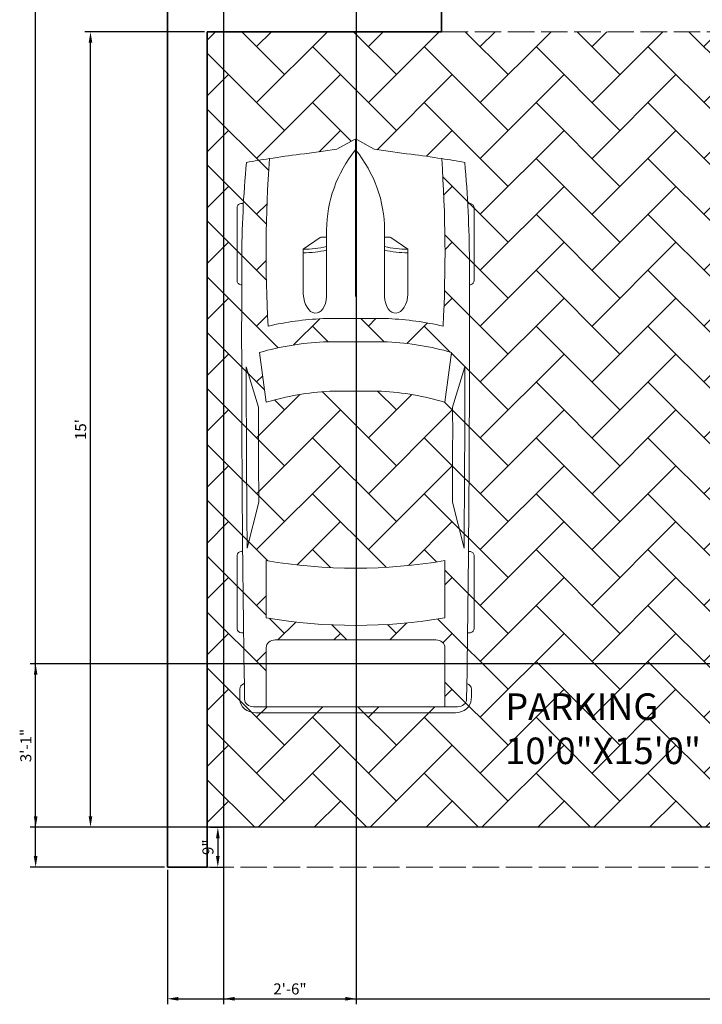
# Model space of a CAD drawing. Units: inches. Extents: x 3889 to 4254, y 3310 to 3958.
# Tile 1 of 6: x 3891 to 4046, y 3311 to 3534. Entities that reach past the tile are written whole.
import ezdxf

# ---------------------------------------------------------------- set-up
doc = ezdxf.new("R2010")
doc.units = ezdxf.units.IN
doc.linetypes.add('ACAD_ISO02W100', pattern=[15, 12, -3])
for name, color, linetype, lineweight in [('A-AREA-IDEN', 11, 'Continuous', 18), ('A-FLOR-OVHD', 7, 'ACAD_ISO02W100', 18), ('A-WALL', 7, 'Continuous', 35), ('CAR', 20, 'Continuous', 13), ('DIM', 81, 'Continuous', 18), ('FLOOR', 7, 'Continuous', 25)]:
    doc.layers.add(name, color=color, linetype=linetype, lineweight=lineweight)
doc.layers.add('A-FLOR-PATT', color=215, linetype='Continuous', lineweight=13, true_color=0xa953a0)
doc.styles.get("Standard").update_dxf_attribs({"font": 'arial.ttf'})
doc.dimstyles.new('ISO-25', dxfattribs={"dimtxt": 2.5, "dimasz": 2.5, "dimexe": 1.25, "dimexo": 0.625, "dimtad": 1, "dimlunit": 3, "dimtxsty": 'Standard', "dimcen": 2.5, "dimadec": 0, "dimazin": 0, "dimtfac": 1, "dimtmove": 0, "dimatfit": 3, "dimfxl": 1, "dimarcsym": 0})

# ---------------------------------------------------------------- blocks, each defined once
blk = doc.blocks.new('*U20')
for p, q in [((46.55368679439944, 38.88847654282876), (22.35054758993934, 38.88847654282876)), ((136.6978032355602, 38.88847654282876), (160.90094244002, 38.88847654282867)), ((21.10406751471477, 37.40863046792069), (21.10406751471477, 36.83230215753705)), ((47.80016686962392, 37.39011648242055), (47.80016686962392, 37.40863046792069)), ((87.98532186932616, 31.87120872459877), (74.75900729854769, 35.92175679182955)), ((134.313356548143, 35.6043097713567), (119.2882629232503, 31.77757799177584)), ((135.4513231603356, 37.07354110333037), (135.4513231603356, 37.40863046792069)), ((162.1474225152445, 37.40863046792049), (162.1474225152445, 36.77402019194128)), ((186.4728846989705, -33.49860931502491), (186.4728846989718, 33.49860931502465)), ((188.3990091454065, -32.75868627757393), (188.3990091454077, 32.75868627757058)), ((70.0302824853563, 31.53613089391356), (86.40615155322342, 29.35124891408057)), ((138.4228833961707, 29.35124891408074), (157.2465674415997, 29.35124891408074)), ((186.4728846989718, 29.35124891408083), (167.0083537481071, 29.35124891408083)), ((164.515393597658, 26.39155676426461), (164.5153935976578, -26.39155676426503)), ((32.26591480791686, 11.62530558863241), (36.12873726252356, 17.16961494239206)), ((36.12873726252356, 17.16961494239206), (50.93891189819171, 17.16961494239206)), ((32.12291633764599, 9.505833383620029), (32.12291633764599, 11.15369945057711)), ((58.9167604809788, -10.77488335095668), (58.9167604809788, 10.77488335095617)), ((66.55009204259746, -10.5288681329018), (66.55009204259746, 10.52886813290129)), ((186.4728846989718, -10.5288681329018), (186.4728846989718, 10.52886813290129)), ((29.77279020470884, 9.505833383620029), (51.68362801571248, 9.505833383620029)), ((82.73706193978568, 8.496039918672748), (82.73706193978568, -8.49603991867258)), ((3.266462181856987, 6.128290093440767), (0.1022408397004821, 0.4060708604429806)), ((-4.43e-14, -2.558e-13), (51.68362801571248, -2.558e-13)), ((0.1022408397004821, -0.4060708604432933), (3.266462181856987, -6.128290093441194)), ((29.77279020470884, -9.50583338362054), (51.68362801571248, -9.50583338362054)), ((32.12291633764599, -9.50583338362054), (32.12291633764599, -11.15369945057762)), ((32.26591480791686, -11.62530558863292), (36.12873726252356, -17.16961494239257)), ((36.12873726252356, -17.16961494239257), (50.93891189819171, -17.16961494239257)), ((86.40615155322318, -29.35124891408145), (70.03028248535594, -31.53613089391442)), ((87.98532186932607, -31.87120872459903), (74.7590072985476, -35.92175679182964)), ((134.3133565481428, -35.60430977135721), (119.2882629232503, -31.77757799177618)), ((157.2465674415997, -29.35124891408117), (138.4228833961707, -29.35124891408126)), ((167.008353748107, -29.35124891408126), (186.4728846989707, -29.35124891408108)), ((21.10406751471477, -37.4086304679212), (21.10406751471477, -36.83230215753756)), ((47.80016686962392, -37.39011648242107), (47.80016686962392, -37.4086304679212)), ((135.4513231603355, -37.07354110333088), (135.4513231603355, -37.4086304679212)), ((162.1474225152445, -37.408630467921), (162.1474225152445, -36.77402019194179)), ((46.55368679439944, -38.88847654282927), (22.35054758993934, -38.88847654282927)), ((136.6978032355602, -38.88847654282927), (160.9009424400199, -38.88847654282918))]:
    blk.add_line(p, q)
for centre, major_axis, ratio, start_param, end_param in [((22.35054758993934, 37.40863046792072), (2.08e-14, -1.479846074908118), 0.842303869543976, 3.141592653589776, 4.712388980384677), ((46.55368679439944, 37.40863046792072), (2.2e-14, 1.479846074908118), 0.8423038695439758, -1.570796326794884, 1.73e-14), ((136.6978032355602, 37.40863046792072), (2.357e-13, -1.479846074908118), 0.842303869543976, 3.141592653589603, 4.712388980384554), ((160.90094244002, 37.40863046792052), (5.59e-14, 1.479846074908118), 0.842303869543976, -1.570796326794865, 4.44e-14), ((266.0300214172791, -27.52442688366631), (1.966072e-10, 313.3077612809058), 0.8423038695435284, 1.367075990158062, 1.391760499156098), ((41.19115208863305, -490.8631038926156), (1.294e-13, 528.2339998381949), 0.8423038695439741, 0.0028100083536837, 0.0755983031096952), ((64.48199294511879, -10555.61767587835), (1.907644e-10, 10593.02630634627), 0.842303869543847, -0.0133969486112073, 0.0027970409639888), ((64.4819929449925, -10555.61767590795), (1.9177683e-09, -10591.54646030096), 0.8423038695482963, 3.133765086725325, 3.140440689641252), ((180.6280394947615, 35.8381667808375), (7.4e-14, 2.219769112362114), 0.8423038695439693, -0.0130174256259048, 1.249894140392862), ((64.48199294754608, -10556.35759891604), (1.349839377e-06, 10595.3130398087), 0.8423038681351469, -0.0133969484821159, -0.0130174254969711), ((183.9799245485226, 33.49860931502124), (3e-16, -2.959692149816168), 0.8423038695439952, 1.570796326796048, 3.128195704978389), ((183.9799245485216, 32.75868627756583), (8.56e-14, -5.246425615115243), 0.8423038695439737, 1.570796326795794, 3.128195704978164), ((37.47375371777758, -593.9621830607928), (6.21e-14, -623.32820996736), 0.8423038695439826, 3.09604606856106, 3.200911180495224), ((135.2911776514449, 5.387441675478555), (2.2715e-12, 81.77258453065997), 0.8423038695439563, 1.245306111696802, 1.507880129813836), ((149.595361812917, 2.799442537139299), (8.561e-13, -79.57966406425402), 0.842303869543983, 4.372215489277867, 4.640744122441986), ((95.78879860270445, -3666.353346297651), (1.949864e-10, -3698.236159209632), 0.8423038695446962, 3.134048706297306, 3.14409775411291), ((17.08207736189386, -1.421e-13), (6.87e-14, 147.0179238898305), 0.8423038695439764, 4.511394369635731, 4.913383591133647), ((35.90576140732288, -1.421e-13), (6.87e-14, 147.0179238898305), 0.8423038695439764, 4.511394369635731, 4.913383591133647), ((167.0083537481071, 26.39155676426464), (1.394e-13, 2.959692149816236), 0.842303869543976, 5.55e-14, 1.57079632679492), ((259.1750197310735, -27.52442688366614), (1.506617e-10, -305.3028914627677), 0.8423038695443789, 4.528606069860317, 4.561837674556238), ((134.4003789125686, 5.387441675477674), (4.276e-13, -89.7774543484738), 0.84230386954398, 4.44948196380473, 4.652344057257214), ((-204.4946649195746, 52.39684969293512), (4.12053e-11, -250.9602162198571), 0.8423038695441164, 1.385369446298923, 1.434372047871027), ((13.03653510440275, 17.00972444508943), (1.2303e-12, 27.41599049210566), 0.8423038695439277, 4.435146050259648, 4.718221029521873), ((14.20086229321332, 17.00972444508943), (1.2303e-12, 27.41599049210566), 0.8423038695439277, 4.435146050259648, 4.718221029521873), ((50.7902773840875, 13.33772416300607), (6.340077547122382, -0.356608581037027), 0.6038335755719145, -1.39555193967809, 1.581314658479915), ((32.74615637525823, 11.15369945057713), (1.313e-13, 0.7399230374541176), 0.8423038695439091, 0.8797135699495516, 1.570796326795045), ((29.77279020470884, -46.66302566589627), (5.12e-14, 56.16885904951626), 0.842303869543976, 7e-16, 0.5903187773915901), ((0.6232400376122422, -1.421e-13), (1e-16, -0.7399230374541245), 0.842303869543842, 4.131459131953847, 5.293318828815531), ((29.77279020470884, 46.66302566589578), (4.004e-13, 56.16885904951626), 0.8423038695439734, 2.55127387619821, 3.141592653589801), ((-204.4946649195746, -52.39684969293552), (4.02945e-11, 250.9602162198562), 0.8423038695441192, -1.43437204787103, -1.385369446298926), ((13.03653510440275, -17.00972444508983), (1.2568e-12, -27.41599049210552), 0.8423038695439318, 1.564964277657711, 1.848039256919935), ((14.20086229321332, -17.00972444508983), (1.2568e-12, -27.41599049210552), 0.8423038695439318, 1.564964277657711, 1.848039256919935), ((149.5953618129329, -2.799442537137565), (4.0897e-12, -79.57966406427697), 0.8423038695439419, -1.499151468852248, -1.230622835688196), ((32.74615637525823, -11.1536994505777), (1.3e-13, -0.7399230374541176), 0.8423038695439093, 4.712388980384541, 5.403471737230034), ((134.4003789125684, -5.387441675478584), (4.2949e-12, -89.77745434847827), 0.8423038695439354, -1.510751403667474, -1.307889310215002), ((135.2911776514465, -5.387441675480715), (3.2038e-12, -81.77258453066244), 0.8423038695439492, -1.50788012981387, -1.245306111696839), ((259.1750197310694, 27.52442688365929), (1.08535e-11, 305.3028914629043), 0.8423038695439974, 1.721347632622872, 1.754579237318777), ((266.0300214172791, 27.52442688366566), (8.75241e-11, 313.3077612806533), 0.8423038695441819, 1.749832154434603, 1.774516663432659), ((37.47375371777847, 593.9621830607904), (1.1693e-12, -623.3282099673584), 0.8423038695439528, -0.0593185269054384, 0.0455465850287298), ((167.008353748107, -26.39155676426503), (1.02e-14, -2.959692149816192), 0.8423038695439885, 4.712388980384686, 6.283185307179581), ((95.78879860271888, 3666.35334629765), (1.637818e-10, -3698.236159209629), 0.8423038695447546, -0.0025051005232382, 0.007543947292366), ((183.9799245485216, -33.4986093150211), (9.3e-15, 2.959692149816141), 0.8423038695439732, 3.154989602201626, 4.71238898038339), ((183.9799245485177, -32.7586862775633), (2.428e-13, -5.246425615118353), 0.8423038695439808, 0.0133969486110846, 1.570796326792831), ((41.19115208863322, 490.8631038926152), (1.37757e-11, -528.2339998381949), 0.8423038695440652, -0.0755983031097181, -0.0028100083537155), ((22.35054758993934, -37.40863046792117), (2.2e-14, 1.479846074908118), 0.8423038695439758, 1.570796326794908, 3.14159265358981), ((64.48199294495228, 10555.61767590795), (6.117947e-10, 10593.02630637587), 0.8423038695458146, 3.138795612625926, 3.154989602201039), ((46.55368679439944, -37.40863046792117), (2.08e-14, -1.479846074908118), 0.842303869543976, -1.69e-14, 1.570796326794884), ((64.48199294503607, 10555.61767590793), (1.6049794e-09, -10591.54646030094), 0.8423038695397146, 0.0011519639481523, 0.0078275668641468), ((136.6978032355602, -37.40863046792109), (1.56e-14, -1.479846074908162), 0.8423038695440105, -1.570796326794875, -1.27e-14), ((160.9009424400199, -37.408630467921), (1.969e-13, 1.479846074908162), 0.8423038695440109, 3.141592653589951, 4.712388980384771), ((180.6280394947581, -35.83816678083949), (2.274e-13, -2.219769112363032), 0.8423038695439803, -1.249894138785958, 0.0130174256254374), ((64.48199294197605, 10556.3575989598), (9.365289701e-07, 10595.31303985772), 0.8423038705260315, 3.154610079306566, 3.154989602290631)]:
    blk.add_ellipse(centre, major_axis=major_axis, ratio=ratio, start_param=start_param, end_param=end_param)
at = {"extrusion": (0, 0, -1)}
blk.add_ellipse((50.7902773840875, -13.33772416300655), major_axis=(6.340077547122382, 0.3566085810370246), ratio=0.6038335755719145, start_param=-1.39555193967809, end_param=1.581314658479915, dxfattribs=at)
blk = doc.blocks.new('*D24')
at = {"layer": 'Defpoints', "color": 0, "transparency": 16777216}
for p in [(3907.440852367994, 3531.107064218412), (3933.842925972467, 3531.107064218412), (3933.84292597247, 3351.107064218411)]:
    blk.add_point(p, dxfattribs=at)
at = {"layer": 'DIM', "color": 0, "lineweight": -2, "transparency": 16777216}
for p, q in [((3933.217925972467, 3531.107064218412), (3906.190852367994, 3531.107064218412)), ((3907.440852367994, 3353.607064218411), (3907.440852367994, 3528.607064218412)), ((3933.217925972471, 3351.107064218411), (3906.190852367994, 3351.107064218411))]:
    blk.add_line(p, q, dxfattribs=at)
at = {"layer": 'DIM', "color": 0, "transparency": 16777216}
for points in [[(3907.024185701328, 3528.607064218412), (3907.85751903466, 3528.607064218412), (3907.440852367994, 3531.107064218412)], [(3907.024185701328, 3353.607064218411), (3907.85751903466, 3353.607064218411), (3907.440852367994, 3351.107064218411)]]:
    blk.add_solid(points, dxfattribs=at)
at = {"layer": 'DIM', "color": 0, "transparency": 16777216, "insert": (3905.53941989869, 3441.107064218409), "char_height": 2.5, "attachment_point": 5, "rotation": 90}
blk.add_mtext("15'", dxfattribs=at)
blk = doc.blocks.new('*D39')
at = {"layer": 'Defpoints', "color": 0, "transparency": 16777216}
for p in [(3933.84292597247, 3351.107064218411), (3933.84292597247, 3342.107064218411), (3936.237722196534, 3342.107064218411)]:
    blk.add_point(p, dxfattribs=at)
at = {"layer": 'DIM', "color": 0, "lineweight": -2, "transparency": 16777216}
for p, q in [((3934.467925972471, 3351.107064218411), (3937.487722196534, 3351.107064218411)), ((3936.237722196534, 3348.607064218411), (3936.237722196534, 3344.607064218411)), ((3934.467925972471, 3342.107064218411), (3937.487722196534, 3342.107064218411))]:
    blk.add_line(p, q, dxfattribs=at)
at = {"layer": 'DIM', "color": 0, "transparency": 16777216}
for points in [[(3935.821055529867, 3348.607064218411), (3936.6543888632, 3348.607064218411), (3936.237722196534, 3351.107064218411)], [(3935.821055529867, 3344.607064218411), (3936.6543888632, 3344.607064218411), (3936.237722196534, 3342.107064218411)]]:
    blk.add_solid(points, dxfattribs=at)
at = {"layer": 'DIM', "color": 0, "transparency": 16777216, "insert": (3934.336289727229, 3346.607064218409), "char_height": 2.5, "attachment_point": 5, "rotation": 90}
blk.add_mtext('9"', dxfattribs=at)
blk = doc.blocks.new('*D69')
at = {"layer": 'Defpoints', "color": 0, "transparency": 16777216}
for p in [(3895.042926000004, 3388.107064000002), (4080.517868000002, 3388.107064000002), (4080.517868000002, 3351.107064000002)]:
    blk.add_point(p, dxfattribs=at)
at = {"layer": 'DIM', "color": 0, "lineweight": -2, "transparency": 16777216}
for p, q in [((4079.892868000001, 3388.107064000002), (3893.792926000004, 3388.107064000002)), ((3895.042926000004, 3353.607064000002), (3895.042926000004, 3385.607064000002)), ((4079.892868000001, 3351.107064000002), (3893.792926000004, 3351.107064000002))]:
    blk.add_line(p, q, dxfattribs=at)
at = {"layer": 'DIM', "color": 0, "transparency": 16777216}
for points in [[(3894.626259333337, 3385.607064000002), (3895.459592666671, 3385.607064000002), (3895.042926000004, 3388.107064000002)], [(3894.626259333337, 3353.607064000002), (3895.459592666671, 3353.607064000002), (3895.042926000004, 3351.107064000002)]]:
    blk.add_solid(points, dxfattribs=at)
at = {"layer": 'DIM', "color": 0, "transparency": 16777216, "insert": (3893.140640870399, 3369.607064), "char_height": 2.5, "attachment_point": 5, "rotation": 90}
blk.add_mtext('3\'-1"', dxfattribs=at)
blk = doc.blocks.new('*D92')
at = {"layer": 'Defpoints', "color": 0, "transparency": 16777216}
for p in [(3937.545523, 3860.107064), (3967.545523, 3860.107064), (3967.545523, 3312.307064)]:
    blk.add_point(p, dxfattribs=at)
at = {"layer": 'DIM', "color": 0, "lineweight": -2, "transparency": 16777216}
for p, q in [((3937.545523, 3859.482064), (3937.545523, 3311.057064)), ((3967.545523, 3859.482064), (3967.545523, 3311.057064)), ((3940.045523, 3312.307064), (3965.045523, 3312.307064))]:
    blk.add_line(p, q, dxfattribs=at)
at = {"layer": 'DIM', "color": 0, "transparency": 16777216}
for points in [[(3940.045523, 3312.723730666667), (3940.045523, 3311.890397333334), (3937.545523, 3312.307064)], [(3965.045523, 3312.723730666667), (3965.045523, 3311.890397333334), (3967.545523, 3312.307064)]]:
    blk.add_solid(points, dxfattribs=at)
at = {"layer": 'DIM', "color": 0, "transparency": 16777216, "insert": (3952.545523, 3314.208496469305), "char_height": 2.5, "attachment_point": 5}
blk.add_mtext('2\'-6"', dxfattribs=at)
blk = doc.blocks.new('*D96')
at = {"layer": 'Defpoints', "color": 0, "transparency": 16777216}
for p in [(3924.842926, 3342.107064), (4222.842926000001, 3342.107064), (4222.842926000001, 3312.307064)]:
    blk.add_point(p, dxfattribs=at)
at = {"layer": 'DIM', "color": 0, "lineweight": -2, "transparency": 16777216}
for p, q in [((3924.842926, 3341.482064), (3924.842926, 3311.057064)), ((4222.842926000001, 3341.482064), (4222.842926000001, 3311.057064)), ((3927.342926, 3312.307064), (4220.342925999999, 3312.307064))]:
    blk.add_line(p, q, dxfattribs=at)
at = {"layer": 'DIM', "color": 0, "transparency": 16777216}
for points in [[(3927.342926, 3312.723730666667), (3927.342926, 3311.890397333334), (3924.842926, 3312.307064)], [(4220.342925999999, 3312.723730666667), (4220.342925999999, 3311.890397333334), (4222.842926000001, 3312.307064)]]:
    blk.add_solid(points, dxfattribs=at)
at = {"layer": 'DIM', "color": 0, "transparency": 16777216, "insert": (4073.842926, 3314.208496469305), "char_height": 2.5, "attachment_point": 5}
blk.add_mtext('24\'-10"', dxfattribs=at)
blk = doc.blocks.new('*D97')
at = {"layer": 'Defpoints', "color": 0, "transparency": 16777216}
for p in [(3895.042926000004, 3922.107064000002), (3924.842926000002, 3922.107064000002), (3924.842926000002, 3342.107064000002)]:
    blk.add_point(p, dxfattribs=at)
at = {"layer": 'DIM', "color": 0, "lineweight": -2, "transparency": 16777216}
for p, q in [((3924.217926000002, 3922.107064000002), (3893.792926000004, 3922.107064000002)), ((3895.042926000004, 3344.607064000002), (3895.042926000004, 3919.607064000002)), ((3924.217926000002, 3342.107064000002), (3893.792926000004, 3342.107064000002))]:
    blk.add_line(p, q, dxfattribs=at)
at = {"layer": 'DIM', "color": 0, "transparency": 16777216}
for points in [[(3894.626259333337, 3919.607064000002), (3895.459592666671, 3919.607064000002), (3895.042926000004, 3922.107064000002)], [(3894.626259333337, 3344.607064000002), (3895.459592666671, 3344.607064000002), (3895.042926000004, 3342.107064000002)]]:
    blk.add_solid(points, dxfattribs=at)
at = {"layer": 'DIM', "color": 0, "transparency": 16777216, "insert": (3893.1414935307, 3632.107063999999), "char_height": 2.5, "attachment_point": 5, "rotation": 90}
blk.add_mtext('48\'-4"', dxfattribs=at)

msp = doc.modelspace()

# ---------------------------------------------------------------- hatches: boundary and pattern name
at = {"layer": 'A-FLOR-PATT', "transparency": 33554477}
h = msp.add_hatch(dxfattribs=at)
h.set_pattern_fill('AR-HBONE', color=256, scale=0.088)
h.set_pattern_definition([(45, (0, 0), (0, 12.64420061846537), [26.8224, -8.9408]), (135, (6.322095999999999, 6.322095999999999), (1.3e-15, 12.64420061846537), [26.8224, -8.9408])])
h.paths.add_polyline_path([(4053.651685410539, 3531.10706421841), (3933.84292597247, 3531.10706421841), (3933.84292597247, 3351.107064218409), (4053.651685410539, 3351.107064218409)])
edge = h.paths.add_edge_path(flags=16)
edge.add_ellipse((3558.368430930596, 3480.977407707075), major_axis=(-429.245727607895, 3.9341e-12), ratio=0.8423038695439133, start_angle=177.8014594340454, end_angle=182.8637146078381, ccw=False)
edge.add_ellipse((3971.101661430321, 3414.230324724107), major_axis=(61.82391250447789, 4.0672e-12), ratio=0.8423038695439867, start_angle=72.28004677724631, end_angle=85.91758930884563)
edge.add_line((3974.811643242401, 3466.210999107257), (3959.971715994079, 3466.210999107257))
edge.add_ellipse((3963.68169780616, 3414.230324724108), major_axis=(-61.82391250447643, 5.4125e-12), ratio=0.8423038695439988, start_angle=-85.91758930884484, end_angle=-72.2800467772449)
edge.add_ellipse((4376.414928305883, 3480.977407707074), major_axis=(429.245727607894, 3.122e-13), ratio=0.8423038695439096, start_angle=177.1362853921623, end_angle=182.198540565955, ccw=False)
edge.add_ellipse((3986.34596799432, 3328.306118778165), major_axis=(210.2423084526331, 6.061938e-10), ratio=0.8423038695415174, start_angle=100.20953899697798, end_angle=102.4446272932787, ccw=False)
edge.add_ellipse((3931.309366141712, 3647.605370721232), major_axis=(-172.8200310675869, 1.162063e-10), ratio=0.8423038695446098, start_angle=99.2565660072399, end_angle=102.5549326441757)
edge.add_line((3963.171523530184, 3504.533751716599), (3967.39167961824, 3506.867375686134))
edge.add_line((3967.39167961824, 3506.867375686134), (3971.611835706296, 3504.533751716599))
edge.add_ellipse((4003.473993094768, 3647.605370721232), major_axis=(172.8200310675602, 1.416865e-10), ratio=0.842303869544737, start_angle=257.4450673558156, end_angle=260.7434339927514)
edge.add_ellipse((3948.437391242156, 3328.306118778163), major_axis=(-210.2423084526045, 5.627318e-10), ratio=0.8423038695416417, start_angle=257.555372706708, end_angle=259.7904610030088, ccw=False)
edge = h.paths.add_edge_path(flags=0)
edge.add_line((3979.215280316628, 3481.903633341898), (3979.215280316628, 3471.704826219371))
edge.add_ellipse((3976.57650555975, 3471.807181173204), major_axis=(0.2455732106949973, 4.366000377148552), ratio=0.6038335755719286, start_angle=106.3425919543003, end_angle=270.9979857249738, ccw=False)
edge.add_line((3973.937730802873, 3471.191988509453), (3973.937730802873, 3486.280562022229))
edge.add_ellipse((3935.257879023218, 3486.280562022235), major_axis=(38.67985177965419, 1.0072e-12), ratio=0.8423038695439817, start_angle=-1.4895e-12, end_angle=29.43856959797854)
edge.add_ellipse((3999.525480213263, 3486.280562022235), major_axis=(-38.67985177965465, 1.0674e-12), ratio=0.8423038695439755, start_angle=-29.43856959797812, end_angle=1.5752e-12)
edge.add_line((3960.845628433608, 3486.280562022235), (3960.845628433608, 3471.191988509453))
edge.add_ellipse((3958.20685367673, 3471.807181173204), major_axis=(-0.2455732106993261, 4.366000377148734), ratio=0.6038335755718637, start_angle=89.00201427496972, end_angle=253.6574080456454, ccw=False)
edge.add_line((3955.568078919853, 3471.704826219371), (3955.568078919853, 3481.903633341898))
edge.add_line((3955.568078919853, 3481.903633341898), (3959.527424749886, 3484.66218251402))
edge.add_line((3959.527424749886, 3484.66218251402), (3960.845628433608, 3484.66218251402))
edge.add_line((3960.845628433608, 3484.66218251402), (3960.845628433608, 3486.280562022235))
edge.add_ellipse((3999.525480213263, 3486.280562022235), major_axis=(-38.67985177965465, 1.0674e-12), ratio=0.8423038695439755, start_angle=-29.438569597978073, end_angle=1.5916157281026244e-12, ccw=False)
edge.add_ellipse((3935.257879023218, 3486.280562022235), major_axis=(38.67985177965419, 1.0072e-12), ratio=0.8423038695439817, start_angle=-1.4779288903810084e-12, end_angle=29.43856959797853, ccw=False)
edge.add_line((3973.937730802873, 3486.280562022229), (3973.937730802873, 3484.66218251402))
edge.add_line((3973.937730802873, 3484.66218251402), (3975.255934486595, 3484.66218251402))
edge.add_line((3975.255934486595, 3484.66218251402), (3979.215280316628, 3481.903633341898))
edge = h.paths.add_edge_path(flags=16)
edge.add_line((3989.108568465939, 3458.557836996553), (3987.603981893128, 3447.280837623114))
edge.add_ellipse((3969.319474204681, 3403.766525096956), major_axis=(-54.80135546223751, 1.9351e-11), ratio=0.8423038695437682, start_angle=247.2080851224298, end_angle=265.1299304028844)
edge.add_line((3973.242351508849, 3449.807501771463), (3961.541007727632, 3449.807501771463))
edge.add_ellipse((3965.463885031801, 3403.766525096945), major_axis=(54.80135546225746, 2.54839e-11), ratio=0.8423038695436712, start_angle=94.8700695971091, end_angle=112.7919148775597)
edge.add_line((3947.179377343352, 3447.280837623115), (3945.674790770542, 3458.557836996553))
edge.add_ellipse((3963.681697806158, 3413.616889383451), major_axis=(-56.31147761958903, 7.9683e-12), ratio=0.8423038695441126, start_angle=-85.72257903693782, end_angle=-68.16504620328351, ccw=False)
edge.add_line((3960.141130725496, 3460.954418532457), (3974.642228510984, 3460.954418532457))
edge.add_ellipse((3971.101661430321, 3413.616889383453), major_axis=(56.31147761958859, 1.0519e-11), ratio=0.8423038695440949, start_angle=68.16504620327959, end_angle=85.72257903693401, ccw=False)
edge = h.paths.add_edge_path(flags=16)
edge.add_line((3987.603981893128, 3411.460286666693), (3987.603981893128, 3398.497635810951))
edge.add_ellipse((3967.39167961824, 3482.057182357768), major_axis=(101.241712956966, 6.132e-13), ratio=0.8423038695439417, start_angle=256.4018653097688, end_angle=283.59813469023015, ccw=False)
edge.add_line((3947.179377343352, 3398.497635810951), (3947.179377343352, 3411.460286666693))
edge.add_ellipse((3967.39167961824, 3495.01983321351), major_axis=(101.241712956966, 6.132e-13), ratio=0.8423038695439417, start_angle=256.4018653097688, end_angle=283.5981346902301)
edge = h.paths.add_edge_path(flags=16)
edge.add_ellipse((3985.565833787478, 3391.775326441849), major_axis=(-2.038148105650179, 1.1849e-12), ratio=0.842303869543886, start_angle=180.0000000000333, end_angle=270.0000000000333, ccw=False)
edge.add_line((3987.603981893128, 3391.775326441849), (3987.603981893128, 3378.371365868674))
edge.add_line((3987.603981893128, 3378.371365868674), (3947.179377343353, 3378.371365868674))
edge.add_line((3947.179377343353, 3378.371365868674), (3947.179377343352, 3391.775326441849))
edge.add_ellipse((3949.217525449002, 3391.775326441849), major_axis=(-2.038148105650179, 1.0283e-12), ratio=0.8423038695438863, start_angle=-89.99999999997101, end_angle=2.8990143619012088e-11, ccw=False)
edge.add_line((3949.217525449002, 3393.492066477942), (3985.565833787478, 3393.492066477942))

# ---------------------------------------------------------------- linework, layer by layer
at = {"layer": 'A-FLOR-OVHD', "ltscale": 0.5}
for p, q in [((3986.842925972468, 3531.107064218411), (4053.84292597247, 3531.107064218409)), ((4053.651685410539, 3351.107064218409), (3933.84292597247, 3351.107064218409)), ((3933.842925972469, 3342.10706421841), (4053.651685410539, 3342.10706421841))]:
    msp.add_line(p, q, dxfattribs=at)
at = {"layer": 'A-WALL'}
for p, q in [((3924.842925972469, 3342.10706421841), (3924.842925972469, 3922.10706421841)), ((3986.842925972468, 3531.107064218409), (3986.842925972469, 3610.107064218411)), ((3933.84292597247, 3351.107064218409), (3933.84292597247, 3531.10706421841)), ((3933.84292597247, 3531.10706421841), (3986.842925972468, 3531.107064218409)), ((3933.842925972469, 3351.107064218409), (3933.842925972469, 3342.10706421841)), ((3933.842925972469, 3342.10706421841), (3924.842925972469, 3342.10706421841))]:
    msp.add_line(p, q, dxfattribs=at)
at = {"layer": 'FLOOR'}
for p, q in [((3933.84292597247, 3531.10706421841), (3986.842925972468, 3531.107064218411)), ((3933.84292597247, 3351.107064218409), (3933.84292597247, 3531.10706421841))]:
    msp.add_line(p, q, dxfattribs=at)

# ---------------------------------------------------------------- block references
at = {"layer": 'CAR', "xscale": 0.6886351696329803, "yscale": 0.6886351696329803, "zscale": 0.6886351696329803, "rotation": 270}
msp.add_blockref('*U20', (3967.39167961824, 3506.783152455302), dxfattribs=at)

# ---------------------------------------------------------------- texts
at = {"layer": 'A-AREA-IDEN', "insert": (4001.237637018705, 3381.411622011271), "char_height": 6, "attachment_point": 1}
msp.add_mtext_dynamic_manual_height_columns('PARKING\\P10\'0"X15\'0"', width=76.45479530175726, gutter_width=12.5, heights=[0], dxfattribs=at)

# ---------------------------------------------------------------- dimensions: what is measured, and where the dimension line sits
at = {"layer": 'DIM'}
for base, p1, p2, override, picture, middle in [((3895.042926000004, 3922.107064000002), (3924.842926, 3342.107064), (3924.842926, 3922.107064), {"dimdec": 1, "dimlfac": 1, "dimrnd": 0, "dimzin": 1, "dimdsep": 46, "dimlunit": 4, "dimfrac": 2}, '*D97', (3893.1414935307, 3632.107063999999)), ((3907.440852367994, 3531.107064218412), (3933.842925972469, 3351.107064218409), (3933.842925972466, 3531.107064218411), {"dimclrd": 0, "dimclre": 0, "dimclrt": 0}, '*D24', (3905.53941989869, 3441.107064218409)), ((3895.042926000004, 3388.107064000002), (4080.517868, 3351.107064), (4080.517868, 3388.107064), {"dimdec": 1, "dimlfac": 1, "dimrnd": 0, "dimzin": 1, "dimdsep": 46, "dimlunit": 4, "dimfrac": 2}, '*D69', (3893.140640870399, 3369.607064)), ((3936.237722196534, 3342.107064218411), (3933.842925972469, 3351.107064218409), (3933.842925972469, 3342.10706421841), {"dimclrd": 0, "dimclre": 0, "dimclrt": 0}, '*D39', (3934.336289727229, 3346.607064218409))]:
    dim = msp.add_linear_dim(base=base, p1=p1, p2=p2, angle=90, dimstyle='ISO-25', override=override, dxfattribs=at)
    dim.commit()
    dim.dimension.update_dxf_attribs({"geometry": picture, "text_midpoint": middle})
for base, p1, p2, picture, middle in [((3967.545523, 3312.307064), (3937.545523, 3860.107064), (3967.545523, 3860.107064), '*D92', (3952.545523, 3314.208496469305)), ((4222.842926000001, 3312.307064), (3924.842926, 3342.107064), (4222.842926000001, 3342.107064), '*D96', (4073.842926, 3314.208496469305))]:
    dim = msp.add_linear_dim(base=base, p1=p1, p2=p2, dimstyle='ISO-25', override={"dimdec": 1, "dimlfac": 1, "dimrnd": 0, "dimzin": 1, "dimdsep": 46, "dimlunit": 4, "dimfrac": 2}, dxfattribs=at)
    dim.commit()
    dim.dimension.update_dxf_attribs({"geometry": picture, "text_midpoint": middle})

doc.saveas('drawing.dxf')
